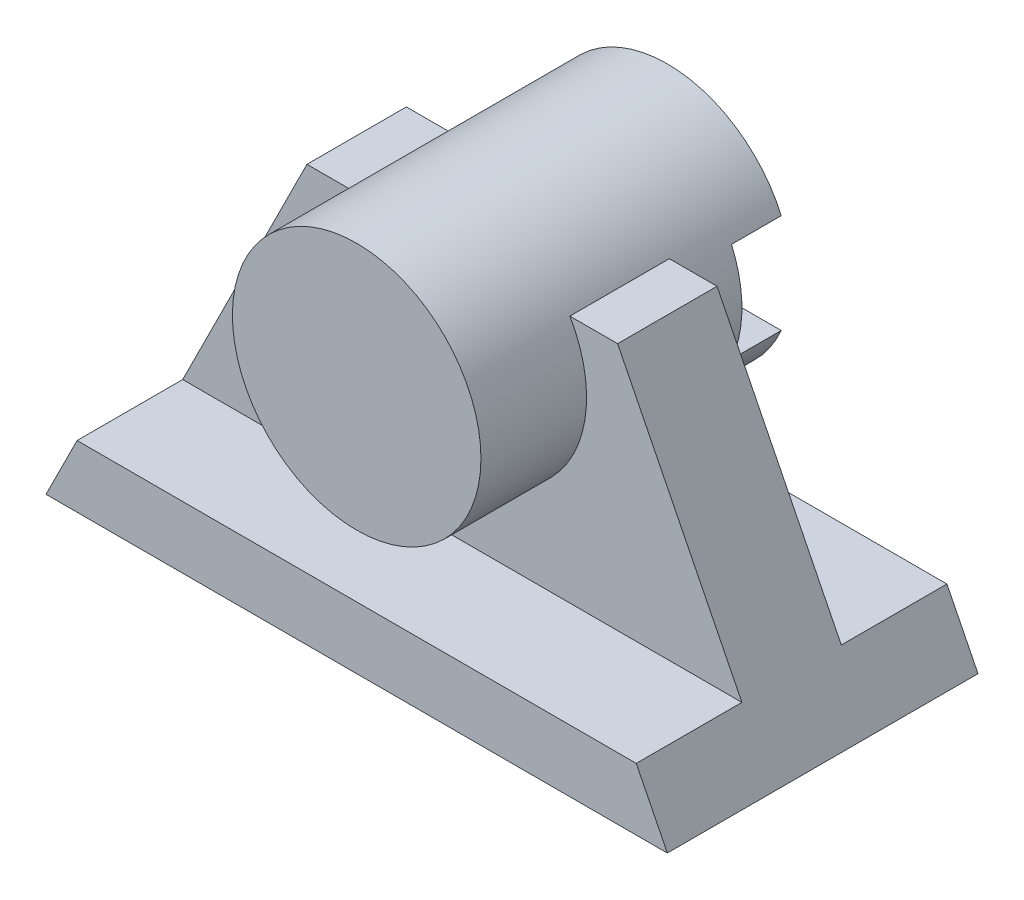
ISO-10303-21;
HEADER;
FILE_DESCRIPTION(('STEP AP214'),'2;1');
FILE_NAME('part.step','',(''),(''),'','','');
FILE_SCHEMA(('AUTOMOTIVE_DESIGN { 1 0 10303 214 1 1 1 1 }'));
ENDSEC;
DATA;
#1=APPLICATION_CONTEXT('core data for automotive mechanical design processes');
#2=APPLICATION_PROTOCOL_DEFINITION('international standard','automotive_design',2000,#1);
#3=PRODUCT_CONTEXT('',#1,'mechanical');
#4=PRODUCT('Part','Part','',(#3));
#5=PRODUCT_RELATED_PRODUCT_CATEGORY('part','',(#4));
#6=PRODUCT_DEFINITION_FORMATION('','',#4);
#7=PRODUCT_DEFINITION_CONTEXT('part definition',#1,'design');
#8=PRODUCT_DEFINITION('design','',#6,#7);
#9=PRODUCT_DEFINITION_SHAPE('','',#8);
#10=(LENGTH_UNIT() NAMED_UNIT(*) SI_UNIT(.MILLI.,.METRE.));
#11=(NAMED_UNIT(*) PLANE_ANGLE_UNIT() SI_UNIT($,.RADIAN.));
#12=(NAMED_UNIT(*) SI_UNIT($,.STERADIAN.) SOLID_ANGLE_UNIT());
#13=UNCERTAINTY_MEASURE_WITH_UNIT(LENGTH_MEASURE(1.E-05),#10,'distance_accuracy_value','');
#14=(GEOMETRIC_REPRESENTATION_CONTEXT(3) GLOBAL_UNCERTAINTY_ASSIGNED_CONTEXT((#13)) GLOBAL_UNIT_ASSIGNED_CONTEXT((#10,
#11,#12)) REPRESENTATION_CONTEXT('',''));
#15=CARTESIAN_POINT('',(0.,0.,0.));
#16=DIRECTION('',(0.,0.,1.));
#17=DIRECTION('',(1.,0.,0.));
#18=AXIS2_PLACEMENT_3D('',#15,#16,#17);
#19=CARTESIAN_POINT('',(50.,40.,-25.));
#20=DIRECTION('',(0.,0.,1.));
#21=DIRECTION('',(1.,0.,0.));
#22=AXIS2_PLACEMENT_3D('',#19,#20,#21);
#23=PLANE('',#22);
#24=CARTESIAN_POINT('',(50.,40.,-25.));
#25=DIRECTION('',(0.,0.,1.));
#26=DIRECTION('',(1.,0.,0.));
#27=AXIS2_PLACEMENT_3D('',#24,#25,#26);
#28=CIRCLE('',#27,20.);
#29=CARTESIAN_POINT('',(68.3303027798234,48.,-25.));
#30=VERTEX_POINT('',#29);
#31=CARTESIAN_POINT('',(31.6696972201766,48.,-25.));
#32=VERTEX_POINT('',#31);
#33=EDGE_CURVE('E172',#30,#32,#28,.T.);
#34=ORIENTED_EDGE('',*,*,#33,.F.);
#35=DIRECTION('',(1.,0.,0.));
#36=VECTOR('',#35,1.);
#37=CARTESIAN_POINT('',(31.6696972201766,48.,-25.));
#38=LINE('',#37,#36);
#39=EDGE_CURVE('E156',#32,#30,#38,.T.);
#40=ORIENTED_EDGE('',*,*,#39,.F.);
#41=EDGE_LOOP('',(#34,#40));
#42=FACE_BOUND('',#41,.T.);
#43=ADVANCED_FACE('F39',(#42),#23,.F.);
#44=CARTESIAN_POINT('',(75.,50.,8.));
#45=DIRECTION('',(0.,-1.,0.));
#46=DIRECTION('',(1.,0.,0.));
#47=AXIS2_PLACEMENT_3D('',#44,#45,#46);
#48=PLANE('',#47);
#49=DIRECTION('',(0.,0.,-1.));
#50=VECTOR('',#49,1.);
#51=CARTESIAN_POINT('',(32.6794919243112,50.,25.));
#52=LINE('',#51,#50);
#53=CARTESIAN_POINT('',(32.6794919243112,50.,-8.));
#54=VERTEX_POINT('',#53);
#55=CARTESIAN_POINT('',(32.6794919243112,50.,8.));
#56=VERTEX_POINT('',#55);
#57=EDGE_CURVE('E180',#54,#56,#52,.F.);
#58=ORIENTED_EDGE('',*,*,#57,.F.);
#59=DIRECTION('',(-1.,0.,0.));
#60=VECTOR('',#59,1.);
#61=CARTESIAN_POINT('',(75.,50.,-8.));
#62=LINE('',#61,#60);
#63=CARTESIAN_POINT('',(25.,50.,-8.));
#64=VERTEX_POINT('',#63);
#65=EDGE_CURVE('E205',#54,#64,#62,.T.);
#66=ORIENTED_EDGE('',*,*,#65,.T.);
#67=DIRECTION('',(0.,0.,-1.));
#68=VECTOR('',#67,1.);
#69=CARTESIAN_POINT('',(25.,50.,8.));
#70=LINE('',#69,#68);
#71=CARTESIAN_POINT('',(25.,50.,8.));
#72=VERTEX_POINT('',#71);
#73=EDGE_CURVE('E192',#72,#64,#70,.T.);
#74=ORIENTED_EDGE('',*,*,#73,.F.);
#75=DIRECTION('',(-1.,0.,0.));
#76=VECTOR('',#75,1.);
#77=CARTESIAN_POINT('',(75.,50.,8.));
#78=LINE('',#77,#76);
#79=EDGE_CURVE('E191',#56,#72,#78,.T.);
#80=ORIENTED_EDGE('',*,*,#79,.F.);
#81=EDGE_LOOP('',(#58,#66,#74,#80));
#82=FACE_BOUND('',#81,.T.);
#83=ADVANCED_FACE('F268',(#82),#48,.F.);
#84=DIRECTION('',(0.,0.,-1.));
#85=VECTOR('',#84,1.);
#86=CARTESIAN_POINT('',(67.3205080756888,50.,25.));
#87=LINE('',#86,#85);
#88=CARTESIAN_POINT('',(67.3205080756888,50.,8.));
#89=VERTEX_POINT('',#88);
#90=CARTESIAN_POINT('',(67.3205080756888,50.,-8.));
#91=VERTEX_POINT('',#90);
#92=EDGE_CURVE('E174',#89,#91,#87,.T.);
#93=ORIENTED_EDGE('',*,*,#92,.F.);
#94=CARTESIAN_POINT('',(75.,50.,8.));
#95=VERTEX_POINT('',#94);
#96=EDGE_CURVE('E195',#95,#89,#78,.T.);
#97=ORIENTED_EDGE('',*,*,#96,.F.);
#98=DIRECTION('',(0.,0.,-1.));
#99=VECTOR('',#98,1.);
#100=CARTESIAN_POINT('',(75.,50.,8.));
#101=LINE('',#100,#99);
#102=CARTESIAN_POINT('',(75.,50.,-8.));
#103=VERTEX_POINT('',#102);
#104=EDGE_CURVE('E210',#95,#103,#101,.T.);
#105=ORIENTED_EDGE('',*,*,#104,.T.);
#106=EDGE_CURVE('E189',#103,#91,#62,.T.);
#107=ORIENTED_EDGE('',*,*,#106,.T.);
#108=EDGE_LOOP('',(#93,#97,#105,#107));
#109=FACE_BOUND('',#108,.T.);
#110=ADVANCED_FACE('F290',(#109),#48,.F.);
#111=CARTESIAN_POINT('',(95.,10.,25.));
#112=DIRECTION('',(0.,-1.,0.));
#113=DIRECTION('',(1.,0.,0.));
#114=AXIS2_PLACEMENT_3D('',#111,#112,#113);
#115=PLANE('',#114);
#116=DIRECTION('',(1.,0.,0.));
#117=VECTOR('',#116,1.);
#118=CARTESIAN_POINT('',(5.,9.99999999999999,8.));
#119=LINE('',#118,#117);
#120=CARTESIAN_POINT('',(5.,9.99999999999999,8.));
#121=VERTEX_POINT('',#120);
#122=CARTESIAN_POINT('',(95.,10.,8.));
#123=VERTEX_POINT('',#122);
#124=EDGE_CURVE('E188',#121,#123,#119,.T.);
#125=ORIENTED_EDGE('',*,*,#124,.F.);
#126=DIRECTION('',(0.,0.,-1.));
#127=VECTOR('',#126,1.);
#128=CARTESIAN_POINT('',(5.,9.99999999999999,25.));
#129=LINE('',#128,#127);
#130=CARTESIAN_POINT('',(5.,9.99999999999999,25.));
#131=VERTEX_POINT('',#130);
#132=EDGE_CURVE('E234',#131,#121,#129,.T.);
#133=ORIENTED_EDGE('',*,*,#132,.F.);
#134=DIRECTION('',(-1.,0.,0.));
#135=VECTOR('',#134,1.);
#136=CARTESIAN_POINT('',(95.,10.,25.));
#137=LINE('',#136,#135);
#138=CARTESIAN_POINT('',(95.,10.,25.));
#139=VERTEX_POINT('',#138);
#140=EDGE_CURVE('E218',#139,#131,#137,.T.);
#141=ORIENTED_EDGE('',*,*,#140,.F.);
#142=DIRECTION('',(0.,0.,-1.));
#143=VECTOR('',#142,1.);
#144=CARTESIAN_POINT('',(95.,10.,25.));
#145=LINE('',#144,#143);
#146=EDGE_CURVE('E232',#139,#123,#145,.T.);
#147=ORIENTED_EDGE('',*,*,#146,.T.);
#148=EDGE_LOOP('',(#125,#133,#141,#147));
#149=FACE_BOUND('',#148,.T.);
#150=ADVANCED_FACE('F279',(#149),#115,.F.);
#151=CARTESIAN_POINT('',(5.,9.99999999999999,25.));
#152=DIRECTION('',(0.894427190999916,-0.447213595499958,0.));
#153=DIRECTION('',(0.447213595499958,0.894427190999916,0.));
#154=AXIS2_PLACEMENT_3D('',#151,#152,#153);
#155=PLANE('',#154);
#156=DIRECTION('',(-0.447213595499958,-0.894427190999916,0.));
#157=VECTOR('',#156,1.);
#158=CARTESIAN_POINT('',(5.,9.99999999999999,-25.));
#159=LINE('',#158,#157);
#160=CARTESIAN_POINT('',(5.,9.99999999999999,-25.));
#161=VERTEX_POINT('',#160);
#162=CARTESIAN_POINT('',(0.,0.,-25.));
#163=VERTEX_POINT('',#162);
#164=EDGE_CURVE('E209',#161,#163,#159,.T.);
#165=ORIENTED_EDGE('',*,*,#164,.T.);
#166=DIRECTION('',(0.,0.,-1.));
#167=VECTOR('',#166,1.);
#168=CARTESIAN_POINT('',(0.,0.,25.));
#169=LINE('',#168,#167);
#170=CARTESIAN_POINT('',(0.,0.,25.));
#171=VERTEX_POINT('',#170);
#172=EDGE_CURVE('E50',#171,#163,#169,.T.);
#173=ORIENTED_EDGE('',*,*,#172,.F.);
#174=DIRECTION('',(-0.447213595499958,-0.894427190999916,0.));
#175=VECTOR('',#174,1.);
#176=CARTESIAN_POINT('',(5.,9.99999999999999,25.));
#177=LINE('',#176,#175);
#178=EDGE_CURVE('E211',#131,#171,#177,.T.);
#179=ORIENTED_EDGE('',*,*,#178,.F.);
#180=ORIENTED_EDGE('',*,*,#132,.T.);
#181=DIRECTION('',(-0.447213595499958,-0.894427190999916,0.));
#182=VECTOR('',#181,1.);
#183=CARTESIAN_POINT('',(25.,50.,8.));
#184=LINE('',#183,#182);
#185=EDGE_CURVE('E181',#72,#121,#184,.T.);
#186=ORIENTED_EDGE('',*,*,#185,.F.);
#187=ORIENTED_EDGE('',*,*,#73,.T.);
#188=DIRECTION('',(-0.447213595499958,-0.894427190999916,0.));
#189=VECTOR('',#188,1.);
#190=CARTESIAN_POINT('',(25.,50.,-8.));
#191=LINE('',#190,#189);
#192=CARTESIAN_POINT('',(5.,9.99999999999999,-8.));
#193=VERTEX_POINT('',#192);
#194=EDGE_CURVE('E185',#64,#193,#191,.T.);
#195=ORIENTED_EDGE('',*,*,#194,.T.);
#196=EDGE_CURVE('E222',#193,#161,#129,.T.);
#197=ORIENTED_EDGE('',*,*,#196,.T.);
#198=EDGE_LOOP('',(#165,#173,#179,#180,#186,#187,#195,#197));
#199=FACE_BOUND('',#198,.T.);
#200=ADVANCED_FACE('F41',(#199),#155,.F.);
#201=CARTESIAN_POINT('',(0.,0.,25.));
#202=DIRECTION('',(0.,1.,0.));
#203=DIRECTION('',(0.,0.,1.));
#204=AXIS2_PLACEMENT_3D('',#201,#202,#203);
#205=PLANE('',#204);
#206=DIRECTION('',(1.,0.,0.));
#207=VECTOR('',#206,1.);
#208=CARTESIAN_POINT('',(0.,0.,-25.));
#209=LINE('',#208,#207);
#210=CARTESIAN_POINT('',(100.,0.,-25.));
#211=VERTEX_POINT('',#210);
#212=EDGE_CURVE('E221',#163,#211,#209,.T.);
#213=ORIENTED_EDGE('',*,*,#212,.T.);
#214=DIRECTION('',(0.,0.,-1.));
#215=VECTOR('',#214,1.);
#216=CARTESIAN_POINT('',(100.,0.,25.));
#217=LINE('',#216,#215);
#218=CARTESIAN_POINT('',(100.,0.,25.));
#219=VERTEX_POINT('',#218);
#220=EDGE_CURVE('E240',#219,#211,#217,.T.);
#221=ORIENTED_EDGE('',*,*,#220,.F.);
#222=DIRECTION('',(1.,0.,0.));
#223=VECTOR('',#222,1.);
#224=CARTESIAN_POINT('',(0.,0.,25.));
#225=LINE('',#224,#223);
#226=EDGE_CURVE('E212',#171,#219,#225,.T.);
#227=ORIENTED_EDGE('',*,*,#226,.F.);
#228=ORIENTED_EDGE('',*,*,#172,.T.);
#229=EDGE_LOOP('',(#213,#221,#227,#228));
#230=FACE_BOUND('',#229,.T.);
#231=ADVANCED_FACE('F244',(#230),#205,.F.);
#232=CARTESIAN_POINT('',(100.,0.,25.));
#233=DIRECTION('',(-0.894427190999916,-0.447213595499958,0.));
#234=DIRECTION('',(0.447213595499958,-0.894427190999916,0.));
#235=AXIS2_PLACEMENT_3D('',#232,#233,#234);
#236=PLANE('',#235);
#237=DIRECTION('',(-0.447213595499958,0.894427190999916,0.));
#238=VECTOR('',#237,1.);
#239=CARTESIAN_POINT('',(100.,0.,-25.));
#240=LINE('',#239,#238);
#241=CARTESIAN_POINT('',(95.,10.,-25.));
#242=VERTEX_POINT('',#241);
#243=EDGE_CURVE('E228',#211,#242,#240,.T.);
#244=ORIENTED_EDGE('',*,*,#243,.T.);
#245=CARTESIAN_POINT('',(95.,10.,-8.));
#246=VERTEX_POINT('',#245);
#247=EDGE_CURVE('E233',#246,#242,#145,.T.);
#248=ORIENTED_EDGE('',*,*,#247,.F.);
#249=DIRECTION('',(-0.447213595499958,0.894427190999916,0.));
#250=VECTOR('',#249,1.);
#251=CARTESIAN_POINT('',(95.,10.,-8.));
#252=LINE('',#251,#250);
#253=EDGE_CURVE('E199',#246,#103,#252,.T.);
#254=ORIENTED_EDGE('',*,*,#253,.T.);
#255=ORIENTED_EDGE('',*,*,#104,.F.);
#256=DIRECTION('',(-0.447213595499958,0.894427190999916,0.));
#257=VECTOR('',#256,1.);
#258=CARTESIAN_POINT('',(95.,10.,8.));
#259=LINE('',#258,#257);
#260=EDGE_CURVE('E186',#123,#95,#259,.T.);
#261=ORIENTED_EDGE('',*,*,#260,.F.);
#262=ORIENTED_EDGE('',*,*,#146,.F.);
#263=DIRECTION('',(-0.447213595499958,0.894427190999916,0.));
#264=VECTOR('',#263,1.);
#265=CARTESIAN_POINT('',(100.,0.,25.));
#266=LINE('',#265,#264);
#267=EDGE_CURVE('E220',#219,#139,#266,.T.);
#268=ORIENTED_EDGE('',*,*,#267,.F.);
#269=ORIENTED_EDGE('',*,*,#220,.T.);
#270=EDGE_LOOP('',(#244,#248,#254,#255,#261,#262,#268,#269));
#271=FACE_BOUND('',#270,.T.);
#272=ADVANCED_FACE('F251',(#271),#236,.F.);
#273=ORIENTED_EDGE('',*,*,#196,.F.);
#274=DIRECTION('',(1.,0.,0.));
#275=VECTOR('',#274,1.);
#276=CARTESIAN_POINT('',(5.,9.99999999999999,-8.));
#277=LINE('',#276,#275);
#278=EDGE_CURVE('E196',#193,#246,#277,.T.);
#279=ORIENTED_EDGE('',*,*,#278,.T.);
#280=ORIENTED_EDGE('',*,*,#247,.T.);
#281=DIRECTION('',(-1.,0.,0.));
#282=VECTOR('',#281,1.);
#283=CARTESIAN_POINT('',(95.,10.,-25.));
#284=LINE('',#283,#282);
#285=EDGE_CURVE('E214',#242,#161,#284,.T.);
#286=ORIENTED_EDGE('',*,*,#285,.T.);
#287=EDGE_LOOP('',(#273,#279,#280,#286));
#288=FACE_BOUND('',#287,.T.);
#289=ADVANCED_FACE('F274',(#288),#115,.F.);
#290=CARTESIAN_POINT('',(0.,0.,25.));
#291=DIRECTION('',(0.,0.,1.));
#292=DIRECTION('',(1.,0.,0.));
#293=AXIS2_PLACEMENT_3D('',#290,#291,#292);
#294=PLANE('',#293);
#295=ORIENTED_EDGE('',*,*,#178,.T.);
#296=ORIENTED_EDGE('',*,*,#226,.T.);
#297=ORIENTED_EDGE('',*,*,#267,.T.);
#298=ORIENTED_EDGE('',*,*,#140,.T.);
#299=EDGE_LOOP('',(#295,#296,#297,#298));
#300=FACE_BOUND('',#299,.T.);
#301=ADVANCED_FACE('F257',(#300),#294,.T.);
#302=CARTESIAN_POINT('',(0.,0.,-25.));
#303=DIRECTION('',(0.,0.,1.));
#304=DIRECTION('',(1.,0.,0.));
#305=AXIS2_PLACEMENT_3D('',#302,#303,#304);
#306=PLANE('',#305);
#307=ORIENTED_EDGE('',*,*,#164,.F.);
#308=ORIENTED_EDGE('',*,*,#285,.F.);
#309=ORIENTED_EDGE('',*,*,#243,.F.);
#310=ORIENTED_EDGE('',*,*,#212,.F.);
#311=EDGE_LOOP('',(#307,#308,#309,#310));
#312=FACE_BOUND('',#311,.T.);
#313=ADVANCED_FACE('F248',(#312),#306,.F.);
#314=CARTESIAN_POINT('',(0.,0.,8.));
#315=DIRECTION('',(0.,0.,1.));
#316=DIRECTION('',(1.,0.,0.));
#317=AXIS2_PLACEMENT_3D('',#314,#315,#316);
#318=PLANE('',#317);
#319=ORIENTED_EDGE('',*,*,#96,.T.);
#320=CARTESIAN_POINT('',(50.,40.,8.));
#321=DIRECTION('',(0.,0.,1.));
#322=DIRECTION('',(1.,0.,0.));
#323=AXIS2_PLACEMENT_3D('',#320,#321,#322);
#324=CIRCLE('',#323,20.);
#325=EDGE_CURVE('E64',#89,#56,#324,.F.);
#326=ORIENTED_EDGE('',*,*,#325,.T.);
#327=ORIENTED_EDGE('',*,*,#79,.T.);
#328=ORIENTED_EDGE('',*,*,#185,.T.);
#329=ORIENTED_EDGE('',*,*,#124,.T.);
#330=ORIENTED_EDGE('',*,*,#260,.T.);
#331=EDGE_LOOP('',(#319,#326,#327,#328,#329,#330));
#332=FACE_BOUND('',#331,.T.);
#333=ADVANCED_FACE('F262',(#332),#318,.T.);
#334=CARTESIAN_POINT('',(0.,0.,-8.));
#335=DIRECTION('',(0.,0.,1.));
#336=DIRECTION('',(1.,0.,0.));
#337=AXIS2_PLACEMENT_3D('',#334,#335,#336);
#338=PLANE('',#337);
#339=CARTESIAN_POINT('',(50.,40.,-8.));
#340=DIRECTION('',(0.,0.,1.));
#341=DIRECTION('',(1.,0.,0.));
#342=AXIS2_PLACEMENT_3D('',#339,#340,#341);
#343=CIRCLE('',#342,20.);
#344=EDGE_CURVE('E11',#91,#54,#343,.F.);
#345=ORIENTED_EDGE('',*,*,#344,.F.);
#346=ORIENTED_EDGE('',*,*,#106,.F.);
#347=ORIENTED_EDGE('',*,*,#253,.F.);
#348=ORIENTED_EDGE('',*,*,#278,.F.);
#349=ORIENTED_EDGE('',*,*,#194,.F.);
#350=ORIENTED_EDGE('',*,*,#65,.F.);
#351=EDGE_LOOP('',(#345,#346,#347,#348,#349,#350));
#352=FACE_BOUND('',#351,.T.);
#353=ADVANCED_FACE('F275',(#352),#338,.F.);
#354=CARTESIAN_POINT('',(50.,40.,25.));
#355=DIRECTION('',(0.,0.,-1.));
#356=DIRECTION('',(-1.,0.,0.));
#357=AXIS2_PLACEMENT_3D('',#354,#355,#356);
#358=CYLINDRICAL_SURFACE('',#357,20.);
#359=CARTESIAN_POINT('',(50.,40.,-17.));
#360=DIRECTION('',(0.,0.,-1.));
#361=DIRECTION('',(-1.,0.,0.));
#362=AXIS2_PLACEMENT_3D('',#359,#360,#361);
#363=CIRCLE('',#362,20.);
#364=CARTESIAN_POINT('',(68.3303027798234,48.,-17.));
#365=VERTEX_POINT('',#364);
#366=CARTESIAN_POINT('',(68.3303027798234,32.,-17.));
#367=VERTEX_POINT('',#366);
#368=EDGE_CURVE('E150',#365,#367,#363,.T.);
#369=ORIENTED_EDGE('',*,*,#368,.F.);
#370=DIRECTION('',(0.,0.,-1.));
#371=VECTOR('',#370,1.);
#372=CARTESIAN_POINT('',(68.3303027798234,48.,-17.));
#373=LINE('',#372,#371);
#374=EDGE_CURVE('E315',#365,#30,#373,.T.);
#375=ORIENTED_EDGE('',*,*,#374,.T.);
#376=ORIENTED_EDGE('',*,*,#33,.T.);
#377=DIRECTION('',(0.,0.,-1.));
#378=VECTOR('',#377,1.);
#379=CARTESIAN_POINT('',(31.6696972201766,48.,-17.));
#380=LINE('',#379,#378);
#381=CARTESIAN_POINT('',(31.6696972201766,48.,-17.));
#382=VERTEX_POINT('',#381);
#383=EDGE_CURVE('E163',#382,#32,#380,.T.);
#384=ORIENTED_EDGE('',*,*,#383,.F.);
#385=CARTESIAN_POINT('',(50.,40.,-17.));
#386=DIRECTION('',(0.,0.,-1.));
#387=DIRECTION('',(-1.,0.,0.));
#388=AXIS2_PLACEMENT_3D('',#385,#386,#387);
#389=CIRCLE('',#388,20.);
#390=CARTESIAN_POINT('',(31.6696972201766,32.,-17.));
#391=VERTEX_POINT('',#390);
#392=EDGE_CURVE('E148',#391,#382,#389,.T.);
#393=ORIENTED_EDGE('',*,*,#392,.F.);
#394=DIRECTION('',(0.,0.,-1.));
#395=VECTOR('',#394,1.);
#396=CARTESIAN_POINT('',(31.6696972201766,32.,-17.));
#397=LINE('',#396,#395);
#398=CARTESIAN_POINT('',(31.6696972201766,32.,-25.));
#399=VERTEX_POINT('',#398);
#400=EDGE_CURVE('E141',#391,#399,#397,.T.);
#401=ORIENTED_EDGE('',*,*,#400,.T.);
#402=CARTESIAN_POINT('',(68.3303027798234,32.,-25.));
#403=VERTEX_POINT('',#402);
#404=EDGE_CURVE('E165',#399,#403,#28,.T.);
#405=ORIENTED_EDGE('',*,*,#404,.T.);
#406=DIRECTION('',(0.,0.,-1.));
#407=VECTOR('',#406,1.);
#408=CARTESIAN_POINT('',(68.3303027798234,32.,-17.));
#409=LINE('',#408,#407);
#410=EDGE_CURVE('E53',#367,#403,#409,.T.);
#411=ORIENTED_EDGE('',*,*,#410,.F.);
#412=EDGE_LOOP('',(#369,#375,#376,#384,#393,#401,#405,#411));
#413=FACE_BOUND('',#412,.T.);
#414=ORIENTED_EDGE('',*,*,#325,.F.);
#415=ORIENTED_EDGE('',*,*,#92,.T.);
#416=ORIENTED_EDGE('',*,*,#344,.T.);
#417=ORIENTED_EDGE('',*,*,#57,.T.);
#418=EDGE_LOOP('',(#414,#415,#416,#417));
#419=FACE_BOUND('',#418,.T.);
#420=CARTESIAN_POINT('',(50.,40.,25.));
#421=DIRECTION('',(0.,0.,1.));
#422=DIRECTION('',(1.,0.,0.));
#423=AXIS2_PLACEMENT_3D('',#420,#421,#422);
#424=CIRCLE('',#423,20.);
#425=CARTESIAN_POINT('',(70.,40.,25.));
#426=VERTEX_POINT('',#425);
#427=EDGE_CURVE('E166',#426,#426,#424,.T.);
#428=ORIENTED_EDGE('',*,*,#427,.F.);
#429=EDGE_LOOP('',(#428));
#430=FACE_BOUND('',#429,.T.);
#431=ADVANCED_FACE('F157',(#413,#419,#430),#358,.T.);
#432=CARTESIAN_POINT('',(50.,40.,25.));
#433=DIRECTION('',(0.,0.,1.));
#434=DIRECTION('',(1.,0.,0.));
#435=AXIS2_PLACEMENT_3D('',#432,#433,#434);
#436=PLANE('',#435);
#437=ORIENTED_EDGE('',*,*,#427,.T.);
#438=EDGE_LOOP('',(#437));
#439=FACE_BOUND('',#438,.T.);
#440=ADVANCED_FACE('F305',(#439),#436,.T.);
#441=ORIENTED_EDGE('',*,*,#404,.F.);
#442=DIRECTION('',(-1.,0.,0.));
#443=VECTOR('',#442,1.);
#444=CARTESIAN_POINT('',(31.6696972201766,32.,-25.));
#445=LINE('',#444,#443);
#446=EDGE_CURVE('E313',#403,#399,#445,.T.);
#447=ORIENTED_EDGE('',*,*,#446,.F.);
#448=EDGE_LOOP('',(#441,#447));
#449=FACE_BOUND('',#448,.T.);
#450=ADVANCED_FACE('F295',(#449),#23,.F.);
#451=CARTESIAN_POINT('',(31.6696972201766,48.,-17.));
#452=DIRECTION('',(0.,1.,0.));
#453=DIRECTION('',(0.,0.,1.));
#454=AXIS2_PLACEMENT_3D('',#451,#452,#453);
#455=PLANE('',#454);
#456=ORIENTED_EDGE('',*,*,#39,.T.);
#457=ORIENTED_EDGE('',*,*,#374,.F.);
#458=DIRECTION('',(1.,0.,0.));
#459=VECTOR('',#458,1.);
#460=CARTESIAN_POINT('',(31.6696972201766,48.,-17.));
#461=LINE('',#460,#459);
#462=EDGE_CURVE('E153',#382,#365,#461,.T.);
#463=ORIENTED_EDGE('',*,*,#462,.F.);
#464=ORIENTED_EDGE('',*,*,#383,.T.);
#465=EDGE_LOOP('',(#456,#457,#463,#464));
#466=FACE_BOUND('',#465,.T.);
#467=ADVANCED_FACE('F301',(#466),#455,.F.);
#468=CARTESIAN_POINT('',(31.6696972201766,32.,-17.));
#469=DIRECTION('',(0.,-1.,0.));
#470=DIRECTION('',(0.,0.,-1.));
#471=AXIS2_PLACEMENT_3D('',#468,#469,#470);
#472=PLANE('',#471);
#473=ORIENTED_EDGE('',*,*,#446,.T.);
#474=ORIENTED_EDGE('',*,*,#400,.F.);
#475=DIRECTION('',(-1.,0.,0.));
#476=VECTOR('',#475,1.);
#477=CARTESIAN_POINT('',(31.6696972201766,32.,-17.));
#478=LINE('',#477,#476);
#479=EDGE_CURVE('E138',#367,#391,#478,.T.);
#480=ORIENTED_EDGE('',*,*,#479,.F.);
#481=ORIENTED_EDGE('',*,*,#410,.T.);
#482=EDGE_LOOP('',(#473,#474,#480,#481));
#483=FACE_BOUND('',#482,.T.);
#484=ADVANCED_FACE('F143',(#483),#472,.F.);
#485=CARTESIAN_POINT('',(50.,40.,-17.));
#486=DIRECTION('',(0.,0.,-1.));
#487=DIRECTION('',(-1.,0.,0.));
#488=AXIS2_PLACEMENT_3D('',#485,#486,#487);
#489=PLANE('',#488);
#490=ORIENTED_EDGE('',*,*,#368,.T.);
#491=ORIENTED_EDGE('',*,*,#479,.T.);
#492=ORIENTED_EDGE('',*,*,#392,.T.);
#493=ORIENTED_EDGE('',*,*,#462,.T.);
#494=EDGE_LOOP('',(#490,#491,#492,#493));
#495=FACE_BOUND('',#494,.T.);
#496=ADVANCED_FACE('F151',(#495),#489,.T.);
#497=CLOSED_SHELL('',(#43,#83,#110,#150,#200,#231,#272,#289,#301,#313,#333,#353,#431,#440,#450,
#467,#484,#496));
#498=MANIFOLD_SOLID_BREP('B2',#497);
#499=ADVANCED_BREP_SHAPE_REPRESENTATION('',(#18,#498),#14);
#500=SHAPE_DEFINITION_REPRESENTATION(#9,#499);
ENDSEC;
END-ISO-10303-21;
